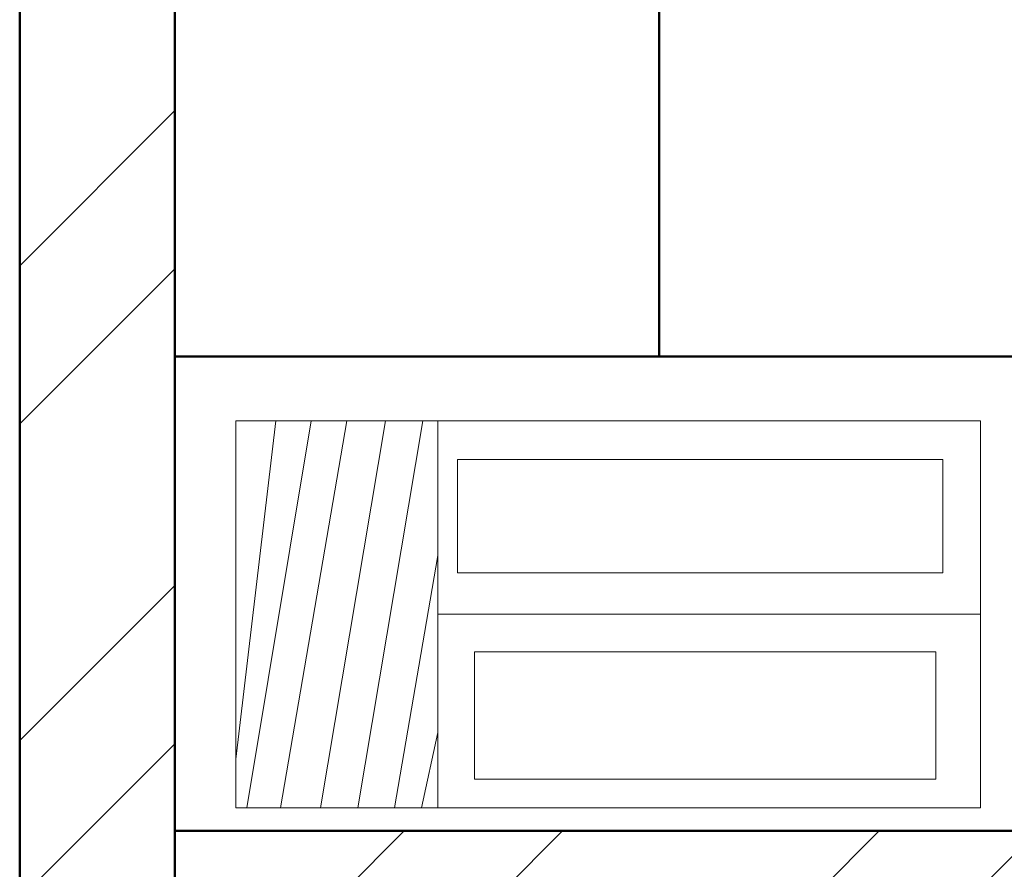
# Model space of a CAD drawing. Units: inches. Extents: x 1901 to 2863, y 888 to 2433.
# Tile 4 of 91: x 2025 to 2053, y 1442 to 1466. Entities that reach past the tile are written whole.
import ezdxf

# ---------------------------------------------------------------- set-up
doc = ezdxf.new("R2010")
doc.units = ezdxf.units.IN
for name, color, linetype, lineweight in [('A-FLOR-FIXT', 9, 'Continuous', 18), ('A-WALL', 7, 'Continuous', 50), ('A-WALL-PATT', 8, 'Continuous', 13)]:
    doc.layers.add(name, color=color, linetype=linetype, lineweight=lineweight)

msp = doc.modelspace()

# ---------------------------------------------------------------- hatches: boundary and pattern name
at = {"layer": 'A-WALL-PATT'}
h = msp.add_hatch(dxfattribs=at)
h.set_pattern_fill('ANSI32', color=256)
h.paths.add_polyline_path([(2182.933, 1716.634), (2024.926, 1716.634), (2024.926, 1681.702), (2029.326, 1681.702), (2029.326, 1712.134), (2154.326, 1712.134), (2154.326, 1580.134), (2148.524, 1580.134), (2148.524, 1577.884), (2148.524, 1575.634), (2194.93, 1575.634), (2194.93, 1580.134), (2158.826, 1580.134), (2158.826, 1712.134), (2182.933, 1712.134)])
h.paths.add_polyline_path([(2301.069, 1716.634), (2242.933, 1716.634), (2242.933, 1712.134), (2283.826, 1712.134), (2283.826, 1685.535), (2288.326, 1685.535), (2288.326, 1712.134), (2301.069, 1712.134)])
h.paths.add_polyline_path([(2288.326, 1600.411), (2286.076, 1600.411), (2283.826, 1600.411), (2283.826, 1580.134), (2270.601, 1580.134), (2270.601, 1575.634), (2288.326, 1575.634)])
h.paths.add_polyline_path([(2295.926, 1953.634), (2271.447, 1953.634), (2271.447, 1949.134), (2291.426, 1949.134), (2291.426, 1941.244), (2295.926, 1941.244)])
h.paths.add_polyline_path([(2098.376, 1244.134), (2082.326, 1244.134), (2082.326, 1302.134), (2086.523, 1302.134), (2086.523, 1306.634), (2067.456, 1306.634), (2067.456, 1302.134), (2077.826, 1302.134), (2077.826, 1239.634), (2098.376, 1239.634), (2098.376, 1241.884)])
h.paths.add_polyline_path([(2217.308, 1306.634), (2158.826, 1306.634), (2158.826, 1451.634), (2162.716, 1451.634), (2162.716, 1453.884), (2162.716, 1456.134), (2154.326, 1456.134), (2154.326, 1443.134), (2151.91, 1443.134), (2151.91, 1438.634), (2154.326, 1438.634), (2154.326, 1306.634), (2109.307, 1306.634), (2109.307, 1304.384), (2109.307, 1302.134), (2154.326, 1302.134), (2154.326, 1244.134), (2122.376, 1244.134), (2122.376, 1239.634), (2154.326, 1239.634), (2154.326, 1223.634), (2163.326, 1223.634), (2181.008, 1223.634), (2181.008, 1225.884), (2181.008, 1228.134), (2163.326, 1228.134), (2163.326, 1258.222), (2158.826, 1258.222), (2158.826, 1302.134), (2217.308, 1302.134)])
h.paths.add_polyline_path([(2259.991, 1306.634), (2238.299, 1306.634), (2238.299, 1304.384), (2238.299, 1302.134), (2242.826, 1302.134), (2242.826, 1228.134), (2205.008, 1228.134), (2205.008, 1223.634), (2247.326, 1223.634), (2247.326, 1302.134), (2259.991, 1302.134), (2259.991, 1304.384)])
h.paths.add_polyline_path([(2343.426, 1361.697), (2338.926, 1361.697), (2338.926, 1306.634), (2322.38, 1306.634), (2322.38, 1302.134), (2343.426, 1302.134)])
h.paths.add_polyline_path([(2343.426, 1470.397), (2338.926, 1470.397), (2338.926, 1456.134), (2193.726, 1456.134), (2193.726, 1453.884), (2193.726, 1451.634), (2338.926, 1451.634), (2338.926, 1421.697), (2343.426, 1421.697)])
h.paths.add_polyline_path([(2343.426, 1545.507), (2338.926, 1545.507), (2338.926, 1530.397), (2343.426, 1530.397)])
h.paths.add_polyline_path([(2029.326, 1466.83), (2024.926, 1466.83), (2024.926, 1409.825), (2029.326, 1409.825)])
h.paths.add_polyline_path([(2122.843, 1440.884), (2122.843, 1443.134), (2121.826, 1443.134), (2121.826, 1498.183), (2119.576, 1498.183), (2117.326, 1498.183), (2117.326, 1443.134), (2029.326, 1443.134), (2029.326, 1438.634), (2122.843, 1438.634)])
h.paths.add_polyline_path([(2029.326, 1543.053), (2024.926, 1543.053), (2024.926, 1502.83), (2029.326, 1502.83)])
h.paths.add_polyline_path([(2029.326, 1621.702), (2024.926, 1621.702), (2024.926, 1567.053), (2027.126, 1567.053), (2029.326, 1567.053), (2029.326, 1575.634), (2109.326, 1575.634), (2109.326, 1554.715), (2113.826, 1554.715), (2113.826, 1575.634), (2115.805, 1575.634), (2115.805, 1577.884), (2115.805, 1580.134), (2029.326, 1580.134)])
h.paths.add_polyline_path([(2121.826, 1527.634), (2117.326, 1527.634), (2113.826, 1527.634), (2113.826, 1533.011), (2111.576, 1533.011), (2109.326, 1533.011), (2109.326, 1527.634), (2029.326, 1527.634), (2029.326, 1523.134), (2117.326, 1523.134), (2117.326, 1519.43), (2121.826, 1519.43)])
h.paths.add_polyline_path([(2029.326, 1349.825), (2024.926, 1349.825), (2024.926, 1302.134), (2036.277, 1302.134), (2036.277, 1306.634), (2029.326, 1306.634)])

# ---------------------------------------------------------------- linework, layer by layer
at = {"layer": 'A-FLOR-FIXT'}
for p, q in [((2032.189, 1454.769), (2031.057, 1445.172)), ((2033.195, 1454.769), (2031.363, 1443.789)), ((2034.202, 1454.769), (2032.189, 1454.769)), ((2034.202, 1454.769), (2032.322, 1443.789)), ((2035.299, 1454.769), (2033.46, 1443.789)), ((2036.355, 1454.769), (2034.512, 1443.789)), ((2036.78, 1454.769), (2036.78, 1443.789)), ((2036.78, 1454.769), (2036.78, 1454.769)), ((2036.78, 1450.951), (2035.556, 1443.789)), ((2036.78, 1449.279), (2052.166, 1449.279)), ((2036.78, 1445.925), (2036.318, 1443.789)), ((2036.004, 1443.789), (2034.202, 1443.789))]:
    msp.add_line(p, q, dxfattribs=at)
for points in [[(2031.057, 1454.769), (2052.166, 1454.769), (2052.166, 1443.789), (2031.057, 1443.789)], [(2037.343, 1453.673), (2051.103, 1453.673), (2051.103, 1450.455), (2037.343, 1450.455)], [(2037.824, 1448.212), (2050.903, 1448.212), (2050.903, 1444.606), (2037.824, 1444.606)]]:
    msp.add_lwpolyline(points, close=True, dxfattribs=at)
at = {"layer": 'A-WALL'}
for p, q in [((2024.926, 1716.634), (2024.926, 1302.134)), ((2029.326, 1575.634), (2029.326, 1306.634)), ((2043.059, 1456.597), (2043.059, 1523.134)), ((2043.059, 1456.597), (2029.326, 1456.597)), ((2117.326, 1456.597), (2043.059, 1456.597)), ((2117.326, 1443.134), (2029.326, 1443.134))]:
    msp.add_line(p, q, dxfattribs=at)

doc.saveas('drawing.dxf')
